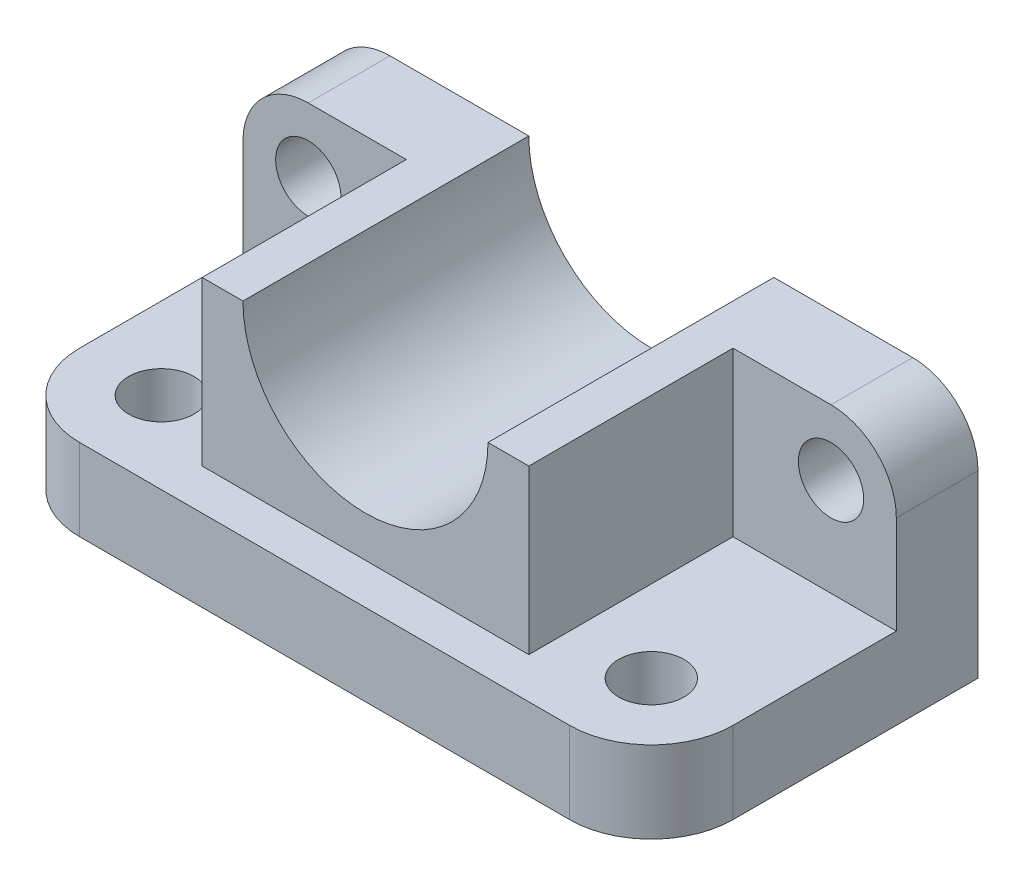
ISO-10303-21;
HEADER;
FILE_DESCRIPTION(('STEP AP214'),'2;1');
FILE_NAME('part.step','',(''),(''),'','','');
FILE_SCHEMA(('AUTOMOTIVE_DESIGN { 1 0 10303 214 1 1 1 1 }'));
ENDSEC;
DATA;
#1=APPLICATION_CONTEXT('core data for automotive mechanical design processes');
#2=APPLICATION_PROTOCOL_DEFINITION('international standard','automotive_design',2000,#1);
#3=PRODUCT_CONTEXT('',#1,'mechanical');
#4=PRODUCT('Part','Part','',(#3));
#5=PRODUCT_RELATED_PRODUCT_CATEGORY('part','',(#4));
#6=PRODUCT_DEFINITION_FORMATION('','',#4);
#7=PRODUCT_DEFINITION_CONTEXT('part definition',#1,'design');
#8=PRODUCT_DEFINITION('design','',#6,#7);
#9=PRODUCT_DEFINITION_SHAPE('','',#8);
#10=(LENGTH_UNIT() NAMED_UNIT(*) SI_UNIT(.MILLI.,.METRE.));
#11=(NAMED_UNIT(*) PLANE_ANGLE_UNIT() SI_UNIT($,.RADIAN.));
#12=(NAMED_UNIT(*) SI_UNIT($,.STERADIAN.) SOLID_ANGLE_UNIT());
#13=UNCERTAINTY_MEASURE_WITH_UNIT(LENGTH_MEASURE(1.E-05),#10,'distance_accuracy_value','');
#14=(GEOMETRIC_REPRESENTATION_CONTEXT(3) GLOBAL_UNCERTAINTY_ASSIGNED_CONTEXT((#13)) GLOBAL_UNIT_ASSIGNED_CONTEXT((#10,
#11,#12)) REPRESENTATION_CONTEXT('',''));
#15=CARTESIAN_POINT('',(0.,0.,0.));
#16=DIRECTION('',(0.,0.,1.));
#17=DIRECTION('',(1.,0.,0.));
#18=AXIS2_PLACEMENT_3D('',#15,#16,#17);
#19=CARTESIAN_POINT('',(0.,10.,0.));
#20=DIRECTION('',(0.,1.,0.));
#21=DIRECTION('',(0.,0.,1.));
#22=AXIS2_PLACEMENT_3D('',#19,#20,#21);
#23=PLANE('',#22);
#24=CARTESIAN_POINT('',(-30.,10.,10.));
#25=DIRECTION('',(0.,1.,0.));
#26=DIRECTION('',(0.,0.,1.));
#27=AXIS2_PLACEMENT_3D('',#24,#25,#26);
#28=CIRCLE('',#27,4.);
#29=CARTESIAN_POINT('',(-30.,10.,14.));
#30=VERTEX_POINT('',#29);
#31=EDGE_CURVE('E261',#30,#30,#28,.T.);
#32=ORIENTED_EDGE('',*,*,#31,.F.);
#33=EDGE_LOOP('',(#32));
#34=FACE_BOUND('',#33,.T.);
#35=CARTESIAN_POINT('',(30.,10.,10.));
#36=DIRECTION('',(0.,1.,0.));
#37=DIRECTION('',(0.,0.,1.));
#38=AXIS2_PLACEMENT_3D('',#35,#36,#37);
#39=CIRCLE('',#38,4.00000000000001);
#40=CARTESIAN_POINT('',(30.,10.,14.));
#41=VERTEX_POINT('',#40);
#42=EDGE_CURVE('E270',#41,#41,#39,.T.);
#43=ORIENTED_EDGE('',*,*,#42,.F.);
#44=EDGE_LOOP('',(#43));
#45=FACE_BOUND('',#44,.T.);
#46=DIRECTION('',(-1.,0.,0.));
#47=VECTOR('',#46,1.);
#48=CARTESIAN_POINT('',(-20.,10.,-10.));
#49=LINE('',#48,#47);
#50=CARTESIAN_POINT('',(-20.,10.,-10.));
#51=VERTEX_POINT('',#50);
#52=CARTESIAN_POINT('',(-40.,10.,-10.));
#53=VERTEX_POINT('',#52);
#54=EDGE_CURVE('E174',#51,#53,#49,.T.);
#55=ORIENTED_EDGE('',*,*,#54,.T.);
#56=DIRECTION('',(0.,0.,1.));
#57=VECTOR('',#56,1.);
#58=CARTESIAN_POINT('',(-40.,10.,-20.));
#59=LINE('',#58,#57);
#60=CARTESIAN_POINT('',(-40.,10.,10.));
#61=VERTEX_POINT('',#60);
#62=EDGE_CURVE('E200',#53,#61,#59,.T.);
#63=ORIENTED_EDGE('',*,*,#62,.T.);
#64=CARTESIAN_POINT('',(-30.,10.,10.));
#65=DIRECTION('',(0.,1.,0.));
#66=DIRECTION('',(0.,0.,1.));
#67=AXIS2_PLACEMENT_3D('',#64,#65,#66);
#68=CIRCLE('',#67,10.);
#69=CARTESIAN_POINT('',(-30.,10.,20.));
#70=VERTEX_POINT('',#69);
#71=EDGE_CURVE('E235',#61,#70,#68,.T.);
#72=ORIENTED_EDGE('',*,*,#71,.T.);
#73=DIRECTION('',(1.,0.,0.));
#74=VECTOR('',#73,1.);
#75=CARTESIAN_POINT('',(-40.,10.,20.));
#76=LINE('',#75,#74);
#77=CARTESIAN_POINT('',(30.,10.,20.));
#78=VERTEX_POINT('',#77);
#79=EDGE_CURVE('E205',#70,#78,#76,.T.);
#80=ORIENTED_EDGE('',*,*,#79,.T.);
#81=CARTESIAN_POINT('',(30.,10.,10.));
#82=DIRECTION('',(0.,1.,0.));
#83=DIRECTION('',(0.,0.,1.));
#84=AXIS2_PLACEMENT_3D('',#81,#82,#83);
#85=CIRCLE('',#84,10.);
#86=CARTESIAN_POINT('',(40.,10.,10.));
#87=VERTEX_POINT('',#86);
#88=EDGE_CURVE('E232',#78,#87,#85,.T.);
#89=ORIENTED_EDGE('',*,*,#88,.T.);
#90=DIRECTION('',(0.,0.,-1.));
#91=VECTOR('',#90,1.);
#92=CARTESIAN_POINT('',(40.,10.,-20.));
#93=LINE('',#92,#91);
#94=CARTESIAN_POINT('',(40.,10.,-10.));
#95=VERTEX_POINT('',#94);
#96=EDGE_CURVE('E198',#87,#95,#93,.T.);
#97=ORIENTED_EDGE('',*,*,#96,.T.);
#98=DIRECTION('',(-1.,0.,0.));
#99=VECTOR('',#98,1.);
#100=CARTESIAN_POINT('',(20.,10.,-10.));
#101=LINE('',#100,#99);
#102=CARTESIAN_POINT('',(20.,10.,-10.));
#103=VERTEX_POINT('',#102);
#104=EDGE_CURVE('E286',#95,#103,#101,.T.);
#105=ORIENTED_EDGE('',*,*,#104,.T.);
#106=DIRECTION('',(0.,0.,-1.));
#107=VECTOR('',#106,1.);
#108=CARTESIAN_POINT('',(20.,10.,15.));
#109=LINE('',#108,#107);
#110=CARTESIAN_POINT('',(20.,10.,15.));
#111=VERTEX_POINT('',#110);
#112=EDGE_CURVE('E189',#111,#103,#109,.T.);
#113=ORIENTED_EDGE('',*,*,#112,.F.);
#114=DIRECTION('',(-1.,0.,0.));
#115=VECTOR('',#114,1.);
#116=CARTESIAN_POINT('',(20.,10.,15.));
#117=LINE('',#116,#115);
#118=CARTESIAN_POINT('',(-20.,10.,15.));
#119=VERTEX_POINT('',#118);
#120=EDGE_CURVE('E294',#111,#119,#117,.T.);
#121=ORIENTED_EDGE('',*,*,#120,.T.);
#122=DIRECTION('',(0.,0.,-1.));
#123=VECTOR('',#122,1.);
#124=CARTESIAN_POINT('',(-20.,10.,15.));
#125=LINE('',#124,#123);
#126=EDGE_CURVE('E184',#119,#51,#125,.T.);
#127=ORIENTED_EDGE('',*,*,#126,.T.);
#128=EDGE_LOOP('',(#55,#63,#72,#80,#89,#97,#105,#113,#121,#127));
#129=FACE_BOUND('',#128,.T.);
#130=ADVANCED_FACE('F43',(#34,#45,#129),#23,.T.);
#131=CARTESIAN_POINT('',(20.,10.,15.));
#132=DIRECTION('',(1.,0.,0.));
#133=DIRECTION('',(0.,0.,-1.));
#134=AXIS2_PLACEMENT_3D('',#131,#132,#133);
#135=PLANE('',#134);
#136=ORIENTED_EDGE('',*,*,#112,.T.);
#137=DIRECTION('',(0.,1.,0.));
#138=VECTOR('',#137,1.);
#139=CARTESIAN_POINT('',(20.,10.,-10.));
#140=LINE('',#139,#138);
#141=CARTESIAN_POINT('',(20.,30.,-10.));
#142=VERTEX_POINT('',#141);
#143=EDGE_CURVE('E176',#103,#142,#140,.T.);
#144=ORIENTED_EDGE('',*,*,#143,.T.);
#145=DIRECTION('',(0.,0.,-1.));
#146=VECTOR('',#145,1.);
#147=CARTESIAN_POINT('',(20.,30.,15.));
#148=LINE('',#147,#146);
#149=CARTESIAN_POINT('',(20.,30.,15.));
#150=VERTEX_POINT('',#149);
#151=EDGE_CURVE('E209',#150,#142,#148,.T.);
#152=ORIENTED_EDGE('',*,*,#151,.F.);
#153=DIRECTION('',(0.,-1.,0.));
#154=VECTOR('',#153,1.);
#155=CARTESIAN_POINT('',(20.,10.,15.));
#156=LINE('',#155,#154);
#157=EDGE_CURVE('E292',#150,#111,#156,.T.);
#158=ORIENTED_EDGE('',*,*,#157,.T.);
#159=EDGE_LOOP('',(#136,#144,#152,#158));
#160=FACE_BOUND('',#159,.T.);
#161=ADVANCED_FACE('F360',(#160),#135,.T.);
#162=CARTESIAN_POINT('',(40.,10.,-20.));
#163=DIRECTION('',(-1.,0.,0.));
#164=DIRECTION('',(0.,0.,1.));
#165=AXIS2_PLACEMENT_3D('',#162,#163,#164);
#166=PLANE('',#165);
#167=DIRECTION('',(0.,-1.,0.));
#168=VECTOR('',#167,1.);
#169=CARTESIAN_POINT('',(40.,10.,-20.));
#170=LINE('',#169,#168);
#171=CARTESIAN_POINT('',(40.,22.,-20.));
#172=VERTEX_POINT('',#171);
#173=CARTESIAN_POINT('',(40.,0.,-20.));
#174=VERTEX_POINT('',#173);
#175=EDGE_CURVE('E218',#172,#174,#170,.T.);
#176=ORIENTED_EDGE('',*,*,#175,.F.);
#177=DIRECTION('',(0.,0.,-1.));
#178=VECTOR('',#177,1.);
#179=CARTESIAN_POINT('',(40.,22.,-10.));
#180=LINE('',#179,#178);
#181=CARTESIAN_POINT('',(40.,22.,-10.));
#182=VERTEX_POINT('',#181);
#183=EDGE_CURVE('E55',#172,#182,#180,.F.);
#184=ORIENTED_EDGE('',*,*,#183,.T.);
#185=DIRECTION('',(0.,-1.,0.));
#186=VECTOR('',#185,1.);
#187=CARTESIAN_POINT('',(40.,10.,-10.));
#188=LINE('',#187,#186);
#189=EDGE_CURVE('E282',#182,#95,#188,.T.);
#190=ORIENTED_EDGE('',*,*,#189,.T.);
#191=ORIENTED_EDGE('',*,*,#96,.F.);
#192=DIRECTION('',(0.,-1.,0.));
#193=VECTOR('',#192,1.);
#194=CARTESIAN_POINT('',(40.,10.,10.));
#195=LINE('',#194,#193);
#196=CARTESIAN_POINT('',(40.,0.,10.));
#197=VERTEX_POINT('',#196);
#198=EDGE_CURVE('E222',#87,#197,#195,.T.);
#199=ORIENTED_EDGE('',*,*,#198,.T.);
#200=DIRECTION('',(0.,0.,-1.));
#201=VECTOR('',#200,1.);
#202=CARTESIAN_POINT('',(40.,0.,-20.));
#203=LINE('',#202,#201);
#204=EDGE_CURVE('E206',#197,#174,#203,.T.);
#205=ORIENTED_EDGE('',*,*,#204,.T.);
#206=EDGE_LOOP('',(#176,#184,#190,#191,#199,#205));
#207=FACE_BOUND('',#206,.T.);
#208=ADVANCED_FACE('F326',(#207),#166,.F.);
#209=CARTESIAN_POINT('',(-40.,10.,-20.));
#210=DIRECTION('',(0.,0.,1.));
#211=DIRECTION('',(1.,0.,0.));
#212=AXIS2_PLACEMENT_3D('',#209,#210,#211);
#213=PLANE('',#212);
#214=CARTESIAN_POINT('',(-32.,22.,-20.));
#215=DIRECTION('',(0.,0.,-1.));
#216=DIRECTION('',(-1.,0.,0.));
#217=AXIS2_PLACEMENT_3D('',#214,#215,#216);
#218=CIRCLE('',#217,4.00000000000001);
#219=CARTESIAN_POINT('',(-36.,22.,-20.));
#220=VERTEX_POINT('',#219);
#221=EDGE_CURVE('E260',#220,#220,#218,.T.);
#222=ORIENTED_EDGE('',*,*,#221,.F.);
#223=EDGE_LOOP('',(#222));
#224=FACE_BOUND('',#223,.T.);
#225=CARTESIAN_POINT('',(32.,22.,-20.));
#226=DIRECTION('',(0.,0.,-1.));
#227=DIRECTION('',(-1.,0.,0.));
#228=AXIS2_PLACEMENT_3D('',#225,#226,#227);
#229=CIRCLE('',#228,4.);
#230=CARTESIAN_POINT('',(28.,22.,-20.));
#231=VERTEX_POINT('',#230);
#232=EDGE_CURVE('E264',#231,#231,#229,.T.);
#233=ORIENTED_EDGE('',*,*,#232,.F.);
#234=EDGE_LOOP('',(#233));
#235=FACE_BOUND('',#234,.T.);
#236=DIRECTION('',(0.,-1.,0.));
#237=VECTOR('',#236,1.);
#238=CARTESIAN_POINT('',(-40.,10.,-20.));
#239=LINE('',#238,#237);
#240=CARTESIAN_POINT('',(-40.,22.,-20.));
#241=VERTEX_POINT('',#240);
#242=CARTESIAN_POINT('',(-40.,0.,-20.));
#243=VERTEX_POINT('',#242);
#244=EDGE_CURVE('E202',#241,#243,#239,.T.);
#245=ORIENTED_EDGE('',*,*,#244,.F.);
#246=CARTESIAN_POINT('',(-32.,22.,-20.));
#247=DIRECTION('',(0.,0.,1.));
#248=DIRECTION('',(1.,0.,0.));
#249=AXIS2_PLACEMENT_3D('',#246,#247,#248);
#250=CIRCLE('',#249,8.);
#251=CARTESIAN_POINT('',(-32.,30.,-20.));
#252=VERTEX_POINT('',#251);
#253=EDGE_CURVE('E242',#241,#252,#250,.F.);
#254=ORIENTED_EDGE('',*,*,#253,.T.);
#255=DIRECTION('',(1.,0.,0.));
#256=VECTOR('',#255,1.);
#257=CARTESIAN_POINT('',(-15.,30.,-20.));
#258=LINE('',#257,#256);
#259=CARTESIAN_POINT('',(-15.,30.,-20.));
#260=VERTEX_POINT('',#259);
#261=EDGE_CURVE('E287',#252,#260,#258,.T.);
#262=ORIENTED_EDGE('',*,*,#261,.T.);
#263=CARTESIAN_POINT('',(0.,30.,-20.));
#264=DIRECTION('',(0.,0.,1.));
#265=DIRECTION('',(-1.,0.,0.));
#266=AXIS2_PLACEMENT_3D('',#263,#264,#265);
#267=CIRCLE('',#266,15.);
#268=CARTESIAN_POINT('',(15.,30.,-20.));
#269=VERTEX_POINT('',#268);
#270=EDGE_CURVE('E307',#260,#269,#267,.T.);
#271=ORIENTED_EDGE('',*,*,#270,.T.);
#272=DIRECTION('',(1.,0.,0.));
#273=VECTOR('',#272,1.);
#274=CARTESIAN_POINT('',(20.,30.,-20.));
#275=LINE('',#274,#273);
#276=CARTESIAN_POINT('',(32.,30.,-20.));
#277=VERTEX_POINT('',#276);
#278=EDGE_CURVE('E293',#269,#277,#275,.T.);
#279=ORIENTED_EDGE('',*,*,#278,.T.);
#280=CARTESIAN_POINT('',(32.,22.,-20.));
#281=DIRECTION('',(0.,0.,1.));
#282=DIRECTION('',(1.,0.,0.));
#283=AXIS2_PLACEMENT_3D('',#280,#281,#282);
#284=CIRCLE('',#283,8.);
#285=EDGE_CURVE('E241',#277,#172,#284,.F.);
#286=ORIENTED_EDGE('',*,*,#285,.T.);
#287=ORIENTED_EDGE('',*,*,#175,.T.);
#288=DIRECTION('',(-1.,0.,0.));
#289=VECTOR('',#288,1.);
#290=CARTESIAN_POINT('',(-40.,0.,-20.));
#291=LINE('',#290,#289);
#292=EDGE_CURVE('E207',#174,#243,#291,.T.);
#293=ORIENTED_EDGE('',*,*,#292,.T.);
#294=EDGE_LOOP('',(#245,#254,#262,#271,#279,#286,#287,#293));
#295=FACE_BOUND('',#294,.T.);
#296=ADVANCED_FACE('F325',(#224,#235,#295),#213,.F.);
#297=CARTESIAN_POINT('',(-40.,10.,-20.));
#298=DIRECTION('',(1.,0.,0.));
#299=DIRECTION('',(0.,0.,-1.));
#300=AXIS2_PLACEMENT_3D('',#297,#298,#299);
#301=PLANE('',#300);
#302=DIRECTION('',(0.,1.,0.));
#303=VECTOR('',#302,1.);
#304=CARTESIAN_POINT('',(-40.,10.,-10.));
#305=LINE('',#304,#303);
#306=CARTESIAN_POINT('',(-40.,22.,-10.));
#307=VERTEX_POINT('',#306);
#308=EDGE_CURVE('E170',#53,#307,#305,.T.);
#309=ORIENTED_EDGE('',*,*,#308,.T.);
#310=DIRECTION('',(0.,0.,-1.));
#311=VECTOR('',#310,1.);
#312=CARTESIAN_POINT('',(-40.,22.,-20.));
#313=LINE('',#312,#311);
#314=EDGE_CURVE('E238',#307,#241,#313,.T.);
#315=ORIENTED_EDGE('',*,*,#314,.T.);
#316=ORIENTED_EDGE('',*,*,#244,.T.);
#317=DIRECTION('',(0.,0.,1.));
#318=VECTOR('',#317,1.);
#319=CARTESIAN_POINT('',(-40.,0.,-20.));
#320=LINE('',#319,#318);
#321=CARTESIAN_POINT('',(-40.,0.,10.));
#322=VERTEX_POINT('',#321);
#323=EDGE_CURVE('E213',#243,#322,#320,.T.);
#324=ORIENTED_EDGE('',*,*,#323,.T.);
#325=DIRECTION('',(0.,-1.,0.));
#326=VECTOR('',#325,1.);
#327=CARTESIAN_POINT('',(-40.,10.,10.));
#328=LINE('',#327,#326);
#329=EDGE_CURVE('E240',#322,#61,#328,.F.);
#330=ORIENTED_EDGE('',*,*,#329,.T.);
#331=ORIENTED_EDGE('',*,*,#62,.F.);
#332=EDGE_LOOP('',(#309,#315,#316,#324,#330,#331));
#333=FACE_BOUND('',#332,.T.);
#334=ADVANCED_FACE('F333',(#333),#301,.F.);
#335=CARTESIAN_POINT('',(-40.,10.,20.));
#336=DIRECTION('',(0.,0.,-1.));
#337=DIRECTION('',(-1.,0.,0.));
#338=AXIS2_PLACEMENT_3D('',#335,#336,#337);
#339=PLANE('',#338);
#340=DIRECTION('',(1.,0.,0.));
#341=VECTOR('',#340,1.);
#342=CARTESIAN_POINT('',(-40.,0.,20.));
#343=LINE('',#342,#341);
#344=CARTESIAN_POINT('',(-30.,0.,20.));
#345=VERTEX_POINT('',#344);
#346=CARTESIAN_POINT('',(30.,0.,20.));
#347=VERTEX_POINT('',#346);
#348=EDGE_CURVE('E199',#345,#347,#343,.T.);
#349=ORIENTED_EDGE('',*,*,#348,.T.);
#350=DIRECTION('',(0.,-1.,0.));
#351=VECTOR('',#350,1.);
#352=CARTESIAN_POINT('',(30.,10.,20.));
#353=LINE('',#352,#351);
#354=EDGE_CURVE('E234',#347,#78,#353,.F.);
#355=ORIENTED_EDGE('',*,*,#354,.T.);
#356=ORIENTED_EDGE('',*,*,#79,.F.);
#357=DIRECTION('',(0.,-1.,0.));
#358=VECTOR('',#357,1.);
#359=CARTESIAN_POINT('',(-30.,10.,20.));
#360=LINE('',#359,#358);
#361=EDGE_CURVE('E226',#70,#345,#360,.T.);
#362=ORIENTED_EDGE('',*,*,#361,.T.);
#363=EDGE_LOOP('',(#349,#355,#356,#362));
#364=FACE_BOUND('',#363,.T.);
#365=ADVANCED_FACE('F349',(#364),#339,.F.);
#366=CARTESIAN_POINT('',(0.,0.,0.));
#367=DIRECTION('',(0.,1.,0.));
#368=DIRECTION('',(0.,0.,1.));
#369=AXIS2_PLACEMENT_3D('',#366,#367,#368);
#370=PLANE('',#369);
#371=CARTESIAN_POINT('',(-30.,0.,10.));
#372=DIRECTION('',(0.,1.,0.));
#373=DIRECTION('',(0.,0.,1.));
#374=AXIS2_PLACEMENT_3D('',#371,#372,#373);
#375=CIRCLE('',#374,4.);
#376=CARTESIAN_POINT('',(-30.,0.,14.));
#377=VERTEX_POINT('',#376);
#378=EDGE_CURVE('E50',#377,#377,#375,.T.);
#379=ORIENTED_EDGE('',*,*,#378,.T.);
#380=EDGE_LOOP('',(#379));
#381=FACE_BOUND('',#380,.T.);
#382=CARTESIAN_POINT('',(30.,0.,10.));
#383=DIRECTION('',(0.,1.,0.));
#384=DIRECTION('',(0.,0.,1.));
#385=AXIS2_PLACEMENT_3D('',#382,#383,#384);
#386=CIRCLE('',#385,4.00000000000001);
#387=CARTESIAN_POINT('',(30.,0.,14.));
#388=VERTEX_POINT('',#387);
#389=EDGE_CURVE('E259',#388,#388,#386,.T.);
#390=ORIENTED_EDGE('',*,*,#389,.T.);
#391=EDGE_LOOP('',(#390));
#392=FACE_BOUND('',#391,.T.);
#393=ORIENTED_EDGE('',*,*,#204,.F.);
#394=CARTESIAN_POINT('',(30.,0.,10.));
#395=DIRECTION('',(0.,1.,0.));
#396=DIRECTION('',(0.,0.,1.));
#397=AXIS2_PLACEMENT_3D('',#394,#395,#396);
#398=CIRCLE('',#397,10.);
#399=EDGE_CURVE('E228',#197,#347,#398,.F.);
#400=ORIENTED_EDGE('',*,*,#399,.T.);
#401=ORIENTED_EDGE('',*,*,#348,.F.);
#402=CARTESIAN_POINT('',(-30.,0.,10.));
#403=DIRECTION('',(0.,1.,0.));
#404=DIRECTION('',(0.,0.,1.));
#405=AXIS2_PLACEMENT_3D('',#402,#403,#404);
#406=CIRCLE('',#405,10.);
#407=EDGE_CURVE('E221',#345,#322,#406,.F.);
#408=ORIENTED_EDGE('',*,*,#407,.T.);
#409=ORIENTED_EDGE('',*,*,#323,.F.);
#410=ORIENTED_EDGE('',*,*,#292,.F.);
#411=EDGE_LOOP('',(#393,#400,#401,#408,#409,#410));
#412=FACE_BOUND('',#411,.T.);
#413=ADVANCED_FACE('F334',(#381,#392,#412),#370,.F.);
#414=CARTESIAN_POINT('',(30.,10.,10.));
#415=DIRECTION('',(0.,-1.,0.));
#416=DIRECTION('',(0.,0.,-1.));
#417=AXIS2_PLACEMENT_3D('',#414,#415,#416);
#418=CYLINDRICAL_SURFACE('',#417,10.);
#419=ORIENTED_EDGE('',*,*,#88,.F.);
#420=ORIENTED_EDGE('',*,*,#354,.F.);
#421=ORIENTED_EDGE('',*,*,#399,.F.);
#422=ORIENTED_EDGE('',*,*,#198,.F.);
#423=EDGE_LOOP('',(#419,#420,#421,#422));
#424=FACE_BOUND('',#423,.T.);
#425=ADVANCED_FACE('F351',(#424),#418,.T.);
#426=CARTESIAN_POINT('',(-30.,10.,10.));
#427=DIRECTION('',(0.,-1.,0.));
#428=DIRECTION('',(0.,0.,-1.));
#429=AXIS2_PLACEMENT_3D('',#426,#427,#428);
#430=CYLINDRICAL_SURFACE('',#429,10.);
#431=ORIENTED_EDGE('',*,*,#71,.F.);
#432=ORIENTED_EDGE('',*,*,#329,.F.);
#433=ORIENTED_EDGE('',*,*,#407,.F.);
#434=ORIENTED_EDGE('',*,*,#361,.F.);
#435=EDGE_LOOP('',(#431,#432,#433,#434));
#436=FACE_BOUND('',#435,.T.);
#437=ADVANCED_FACE('F342',(#436),#430,.T.);
#438=CARTESIAN_POINT('',(20.,30.,15.));
#439=DIRECTION('',(0.,1.,0.));
#440=DIRECTION('',(0.,0.,1.));
#441=AXIS2_PLACEMENT_3D('',#438,#439,#440);
#442=PLANE('',#441);
#443=DIRECTION('',(1.,0.,0.));
#444=VECTOR('',#443,1.);
#445=CARTESIAN_POINT('',(20.,30.,-10.));
#446=LINE('',#445,#444);
#447=CARTESIAN_POINT('',(32.,30.,-10.));
#448=VERTEX_POINT('',#447);
#449=EDGE_CURVE('E281',#142,#448,#446,.T.);
#450=ORIENTED_EDGE('',*,*,#449,.T.);
#451=DIRECTION('',(0.,0.,-1.));
#452=VECTOR('',#451,1.);
#453=CARTESIAN_POINT('',(32.,30.,-20.));
#454=LINE('',#453,#452);
#455=EDGE_CURVE('E247',#448,#277,#454,.T.);
#456=ORIENTED_EDGE('',*,*,#455,.T.);
#457=ORIENTED_EDGE('',*,*,#278,.F.);
#458=DIRECTION('',(0.,0.,-1.));
#459=VECTOR('',#458,1.);
#460=CARTESIAN_POINT('',(15.,30.,15.));
#461=LINE('',#460,#459);
#462=CARTESIAN_POINT('',(15.,30.,15.));
#463=VERTEX_POINT('',#462);
#464=EDGE_CURVE('E190',#463,#269,#461,.T.);
#465=ORIENTED_EDGE('',*,*,#464,.F.);
#466=DIRECTION('',(1.,0.,0.));
#467=VECTOR('',#466,1.);
#468=CARTESIAN_POINT('',(20.,30.,15.));
#469=LINE('',#468,#467);
#470=EDGE_CURVE('E192',#463,#150,#469,.T.);
#471=ORIENTED_EDGE('',*,*,#470,.T.);
#472=ORIENTED_EDGE('',*,*,#151,.T.);
#473=EDGE_LOOP('',(#450,#456,#457,#465,#471,#472));
#474=FACE_BOUND('',#473,.T.);
#475=ADVANCED_FACE('F323',(#474),#442,.T.);
#476=CARTESIAN_POINT('',(0.,30.,15.));
#477=DIRECTION('',(0.,0.,-1.));
#478=DIRECTION('',(-1.,0.,0.));
#479=AXIS2_PLACEMENT_3D('',#476,#477,#478);
#480=CYLINDRICAL_SURFACE('',#479,15.);
#481=ORIENTED_EDGE('',*,*,#270,.F.);
#482=DIRECTION('',(0.,0.,-1.));
#483=VECTOR('',#482,1.);
#484=CARTESIAN_POINT('',(-15.,30.,15.));
#485=LINE('',#484,#483);
#486=CARTESIAN_POINT('',(-15.,30.,15.));
#487=VERTEX_POINT('',#486);
#488=EDGE_CURVE('E181',#487,#260,#485,.T.);
#489=ORIENTED_EDGE('',*,*,#488,.F.);
#490=CARTESIAN_POINT('',(0.,30.,15.));
#491=DIRECTION('',(0.,0.,1.));
#492=DIRECTION('',(-1.,0.,0.));
#493=AXIS2_PLACEMENT_3D('',#490,#491,#492);
#494=CIRCLE('',#493,15.);
#495=EDGE_CURVE('E304',#487,#463,#494,.T.);
#496=ORIENTED_EDGE('',*,*,#495,.T.);
#497=ORIENTED_EDGE('',*,*,#464,.T.);
#498=EDGE_LOOP('',(#481,#489,#496,#497));
#499=FACE_BOUND('',#498,.T.);
#500=ADVANCED_FACE('F312',(#499),#480,.F.);
#501=CARTESIAN_POINT('',(-15.,30.,15.));
#502=DIRECTION('',(0.,1.,0.));
#503=DIRECTION('',(0.,0.,1.));
#504=AXIS2_PLACEMENT_3D('',#501,#502,#503);
#505=PLANE('',#504);
#506=ORIENTED_EDGE('',*,*,#261,.F.);
#507=DIRECTION('',(0.,0.,-1.));
#508=VECTOR('',#507,1.);
#509=CARTESIAN_POINT('',(-32.,30.,-10.));
#510=LINE('',#509,#508);
#511=CARTESIAN_POINT('',(-32.,30.,-10.));
#512=VERTEX_POINT('',#511);
#513=EDGE_CURVE('E163',#252,#512,#510,.F.);
#514=ORIENTED_EDGE('',*,*,#513,.T.);
#515=DIRECTION('',(1.,0.,0.));
#516=VECTOR('',#515,1.);
#517=CARTESIAN_POINT('',(-20.,30.,-10.));
#518=LINE('',#517,#516);
#519=CARTESIAN_POINT('',(-20.,30.,-10.));
#520=VERTEX_POINT('',#519);
#521=EDGE_CURVE('E154',#512,#520,#518,.T.);
#522=ORIENTED_EDGE('',*,*,#521,.T.);
#523=DIRECTION('',(0.,0.,-1.));
#524=VECTOR('',#523,1.);
#525=CARTESIAN_POINT('',(-20.,30.,15.));
#526=LINE('',#525,#524);
#527=CARTESIAN_POINT('',(-20.,30.,15.));
#528=VERTEX_POINT('',#527);
#529=EDGE_CURVE('E161',#528,#520,#526,.T.);
#530=ORIENTED_EDGE('',*,*,#529,.F.);
#531=DIRECTION('',(1.,0.,0.));
#532=VECTOR('',#531,1.);
#533=CARTESIAN_POINT('',(-15.,30.,15.));
#534=LINE('',#533,#532);
#535=EDGE_CURVE('E299',#528,#487,#534,.T.);
#536=ORIENTED_EDGE('',*,*,#535,.T.);
#537=ORIENTED_EDGE('',*,*,#488,.T.);
#538=EDGE_LOOP('',(#506,#514,#522,#530,#536,#537));
#539=FACE_BOUND('',#538,.T.);
#540=ADVANCED_FACE('F158',(#539),#505,.T.);
#541=CARTESIAN_POINT('',(-20.,10.,15.));
#542=DIRECTION('',(-1.,0.,0.));
#543=DIRECTION('',(0.,-1.,0.));
#544=AXIS2_PLACEMENT_3D('',#541,#542,#543);
#545=PLANE('',#544);
#546=DIRECTION('',(0.,-1.,0.));
#547=VECTOR('',#546,1.);
#548=CARTESIAN_POINT('',(-20.,10.,-10.));
#549=LINE('',#548,#547);
#550=EDGE_CURVE('E173',#520,#51,#549,.T.);
#551=ORIENTED_EDGE('',*,*,#550,.T.);
#552=ORIENTED_EDGE('',*,*,#126,.F.);
#553=DIRECTION('',(0.,1.,0.));
#554=VECTOR('',#553,1.);
#555=CARTESIAN_POINT('',(-20.,10.,15.));
#556=LINE('',#555,#554);
#557=EDGE_CURVE('E185',#119,#528,#556,.T.);
#558=ORIENTED_EDGE('',*,*,#557,.T.);
#559=ORIENTED_EDGE('',*,*,#529,.T.);
#560=EDGE_LOOP('',(#551,#552,#558,#559));
#561=FACE_BOUND('',#560,.T.);
#562=ADVANCED_FACE('F177',(#561),#545,.T.);
#563=CARTESIAN_POINT('',(0.,30.,15.));
#564=DIRECTION('',(0.,0.,-1.));
#565=DIRECTION('',(-1.,0.,0.));
#566=AXIS2_PLACEMENT_3D('',#563,#564,#565);
#567=PLANE('',#566);
#568=ORIENTED_EDGE('',*,*,#157,.F.);
#569=ORIENTED_EDGE('',*,*,#470,.F.);
#570=ORIENTED_EDGE('',*,*,#495,.F.);
#571=ORIENTED_EDGE('',*,*,#535,.F.);
#572=ORIENTED_EDGE('',*,*,#557,.F.);
#573=ORIENTED_EDGE('',*,*,#120,.F.);
#574=EDGE_LOOP('',(#568,#569,#570,#571,#572,#573));
#575=FACE_BOUND('',#574,.T.);
#576=ADVANCED_FACE('F363',(#575),#567,.F.);
#577=CARTESIAN_POINT('',(0.,0.,-10.));
#578=DIRECTION('',(0.,0.,-1.));
#579=DIRECTION('',(-1.,0.,0.));
#580=AXIS2_PLACEMENT_3D('',#577,#578,#579);
#581=PLANE('',#580);
#582=CARTESIAN_POINT('',(32.,22.,-9.99999999999999));
#583=DIRECTION('',(0.,0.,-1.));
#584=DIRECTION('',(-1.,0.,0.));
#585=AXIS2_PLACEMENT_3D('',#582,#583,#584);
#586=CIRCLE('',#585,4.);
#587=CARTESIAN_POINT('',(28.,22.,-9.99999999999999));
#588=VERTEX_POINT('',#587);
#589=EDGE_CURVE('E169',#588,#588,#586,.T.);
#590=ORIENTED_EDGE('',*,*,#589,.T.);
#591=EDGE_LOOP('',(#590));
#592=FACE_BOUND('',#591,.T.);
#593=ORIENTED_EDGE('',*,*,#189,.F.);
#594=CARTESIAN_POINT('',(32.,22.,-10.));
#595=DIRECTION('',(0.,0.,-1.));
#596=DIRECTION('',(-1.,0.,0.));
#597=AXIS2_PLACEMENT_3D('',#594,#595,#596);
#598=CIRCLE('',#597,8.);
#599=EDGE_CURVE('E11',#182,#448,#598,.F.);
#600=ORIENTED_EDGE('',*,*,#599,.T.);
#601=ORIENTED_EDGE('',*,*,#449,.F.);
#602=ORIENTED_EDGE('',*,*,#143,.F.);
#603=ORIENTED_EDGE('',*,*,#104,.F.);
#604=EDGE_LOOP('',(#593,#600,#601,#602,#603));
#605=FACE_BOUND('',#604,.T.);
#606=ADVANCED_FACE('F352',(#592,#605),#581,.F.);
#607=CARTESIAN_POINT('',(0.,0.,-10.));
#608=DIRECTION('',(0.,0.,1.));
#609=DIRECTION('',(1.,0.,0.));
#610=AXIS2_PLACEMENT_3D('',#607,#608,#609);
#611=PLANE('',#610);
#612=CARTESIAN_POINT('',(-32.,22.,-9.99999999999999));
#613=DIRECTION('',(0.,0.,1.));
#614=DIRECTION('',(1.,0.,0.));
#615=AXIS2_PLACEMENT_3D('',#612,#613,#614);
#616=CIRCLE('',#615,4.00000000000001);
#617=CARTESIAN_POINT('',(-28.,22.,-9.99999999999999));
#618=VERTEX_POINT('',#617);
#619=EDGE_CURVE('E255',#618,#618,#616,.T.);
#620=ORIENTED_EDGE('',*,*,#619,.F.);
#621=EDGE_LOOP('',(#620));
#622=FACE_BOUND('',#621,.T.);
#623=ORIENTED_EDGE('',*,*,#521,.F.);
#624=CARTESIAN_POINT('',(-32.,22.,-10.));
#625=DIRECTION('',(0.,0.,1.));
#626=DIRECTION('',(1.,0.,0.));
#627=AXIS2_PLACEMENT_3D('',#624,#625,#626);
#628=CIRCLE('',#627,8.);
#629=EDGE_CURVE('E250',#512,#307,#628,.T.);
#630=ORIENTED_EDGE('',*,*,#629,.T.);
#631=ORIENTED_EDGE('',*,*,#308,.F.);
#632=ORIENTED_EDGE('',*,*,#54,.F.);
#633=ORIENTED_EDGE('',*,*,#550,.F.);
#634=EDGE_LOOP('',(#623,#630,#631,#632,#633));
#635=FACE_BOUND('',#634,.T.);
#636=ADVANCED_FACE('F175',(#622,#635),#611,.T.);
#637=CARTESIAN_POINT('',(-32.,22.,-20.));
#638=DIRECTION('',(0.,0.,1.));
#639=DIRECTION('',(1.,0.,0.));
#640=AXIS2_PLACEMENT_3D('',#637,#638,#639);
#641=CYLINDRICAL_SURFACE('',#640,8.);
#642=ORIENTED_EDGE('',*,*,#629,.F.);
#643=ORIENTED_EDGE('',*,*,#513,.F.);
#644=ORIENTED_EDGE('',*,*,#253,.F.);
#645=ORIENTED_EDGE('',*,*,#314,.F.);
#646=EDGE_LOOP('',(#642,#643,#644,#645));
#647=FACE_BOUND('',#646,.T.);
#648=ADVANCED_FACE('F337',(#647),#641,.T.);
#649=CARTESIAN_POINT('',(32.,22.,15.));
#650=DIRECTION('',(0.,0.,1.));
#651=DIRECTION('',(1.,0.,0.));
#652=AXIS2_PLACEMENT_3D('',#649,#650,#651);
#653=CYLINDRICAL_SURFACE('',#652,8.);
#654=ORIENTED_EDGE('',*,*,#599,.F.);
#655=ORIENTED_EDGE('',*,*,#183,.F.);
#656=ORIENTED_EDGE('',*,*,#285,.F.);
#657=ORIENTED_EDGE('',*,*,#455,.F.);
#658=EDGE_LOOP('',(#654,#655,#656,#657));
#659=FACE_BOUND('',#658,.T.);
#660=ADVANCED_FACE('F44',(#659),#653,.T.);
#661=CARTESIAN_POINT('',(-32.,22.,42.));
#662=DIRECTION('',(0.,0.,-1.));
#663=DIRECTION('',(-1.,0.,0.));
#664=AXIS2_PLACEMENT_3D('',#661,#662,#663);
#665=CYLINDRICAL_SURFACE('',#664,4.00000000000001);
#666=ORIENTED_EDGE('',*,*,#619,.T.);
#667=EDGE_LOOP('',(#666));
#668=FACE_BOUND('',#667,.T.);
#669=ORIENTED_EDGE('',*,*,#221,.T.);
#670=EDGE_LOOP('',(#669));
#671=FACE_BOUND('',#670,.T.);
#672=ADVANCED_FACE('F405',(#668,#671),#665,.F.);
#673=CARTESIAN_POINT('',(32.,22.,42.));
#674=DIRECTION('',(0.,0.,-1.));
#675=DIRECTION('',(-1.,0.,0.));
#676=AXIS2_PLACEMENT_3D('',#673,#674,#675);
#677=CYLINDRICAL_SURFACE('',#676,4.);
#678=ORIENTED_EDGE('',*,*,#232,.T.);
#679=EDGE_LOOP('',(#678));
#680=FACE_BOUND('',#679,.T.);
#681=ORIENTED_EDGE('',*,*,#589,.F.);
#682=EDGE_LOOP('',(#681));
#683=FACE_BOUND('',#682,.T.);
#684=ADVANCED_FACE('F414',(#680,#683),#677,.F.);
#685=CARTESIAN_POINT('',(30.,-52.,10.));
#686=DIRECTION('',(0.,1.,0.));
#687=DIRECTION('',(0.,0.,1.));
#688=AXIS2_PLACEMENT_3D('',#685,#686,#687);
#689=CYLINDRICAL_SURFACE('',#688,4.00000000000001);
#690=ORIENTED_EDGE('',*,*,#42,.T.);
#691=EDGE_LOOP('',(#690));
#692=FACE_BOUND('',#691,.T.);
#693=ORIENTED_EDGE('',*,*,#389,.F.);
#694=EDGE_LOOP('',(#693));
#695=FACE_BOUND('',#694,.T.);
#696=ADVANCED_FACE('F413',(#692,#695),#689,.F.);
#697=CARTESIAN_POINT('',(-30.,-52.,10.));
#698=DIRECTION('',(0.,1.,0.));
#699=DIRECTION('',(0.,0.,1.));
#700=AXIS2_PLACEMENT_3D('',#697,#698,#699);
#701=CYLINDRICAL_SURFACE('',#700,4.);
#702=ORIENTED_EDGE('',*,*,#31,.T.);
#703=EDGE_LOOP('',(#702));
#704=FACE_BOUND('',#703,.T.);
#705=ORIENTED_EDGE('',*,*,#378,.F.);
#706=EDGE_LOOP('',(#705));
#707=FACE_BOUND('',#706,.T.);
#708=ADVANCED_FACE('F419',(#704,#707),#701,.F.);
#709=CLOSED_SHELL('',(#130,#161,#208,#296,#334,#365,#413,#425,#437,#475,#500,#540,#562,#576,
#606,#636,#648,#660,#672,#684,#696,#708));
#710=MANIFOLD_SOLID_BREP('B2',#709);
#711=ADVANCED_BREP_SHAPE_REPRESENTATION('',(#18,#710),#14);
#712=SHAPE_DEFINITION_REPRESENTATION(#9,#711);
ENDSEC;
END-ISO-10303-21;
